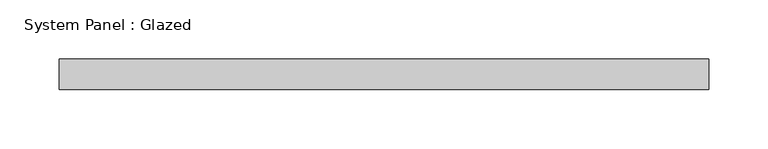
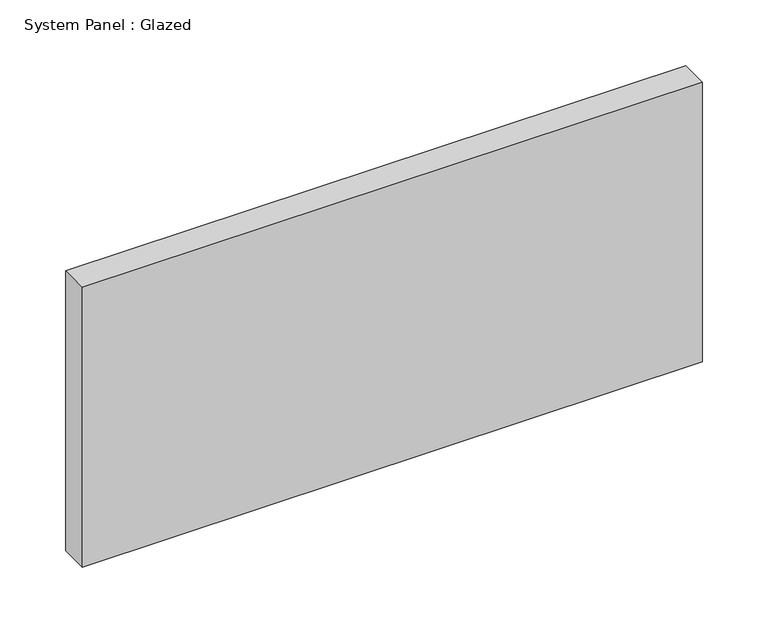
"""IFC4 building model written with IfcOpenShell, lengths in millimetres: plate geometry, System Panel : Glazed."""

from ifc_helpers import new_model, si_unit, origin, origin_with_axes, place, context, project, spatial, polyline, outline, extrude, source, transform, mapped, element, save


def system_panel_glazed_6ade1748(model_context):
    return source(origin(), model_context, "Body", "SweptSolid", [
        extrude(outline(polyline([(273.05, 19.05), (-273.05, 19.05), (-273.05, 44.45), (273.05, 44.45), (273.05, 19.05)])), origin_with_axes(), (0.0, 0.0, 1.0), 260.35),
    ])


if __name__ == "__main__":
    model = new_model("IFC4")
    model_context = context("Model", 3, world=origin())
    ifc_project = project(units=[si_unit("LENGTHUNIT", "METRE", prefix="MILLI")], contexts=[model_context])
    site = spatial("IfcSite", under=ifc_project)
    building = spatial("IfcBuilding", under=site)
    placement = place(None, origin())
    system_panel_glazed_shape = system_panel_glazed_6ade1748(model_context)
    element("IfcPlate", 1, ObjectType="System Panel : Glazed", at=placement, inside=building, context=model_context, shape_type="MappedRepresentation", body=[
        mapped(system_panel_glazed_shape, transform((0.0, 0.0, 0.0), x_axis=(1.0, 0.0, 0.0), y_axis=(0.0, 1.0, 0.0), z_axis=(0.0, 0.0, 1.0))),
    ])
    save(model, "model.ifc")

# Revit data of these elements
# Type "System Panel : Glazed"
#   Construction Type Id = "GSP4R"
#   Analytic Construction = "1/8 in Pilkington single glazing"
#   Visual Light Transmittance = 0.9
#   Solar Heat Gain Coefficient = 0.86
#   Heat Transfer Coefficient (U) = 1.18115 BTU/(h·ft²·°F)
#   Define Thermal Properties by = 1
# Element 1 (IfcPlate, "System Panel : Glazed")
#   Materials on its faces: "Glass"
# Materials
#   "Glass": class "Glass", colour RGB 0 128 192, transparency 0.75, Description = "Soda Lime Glass", Cost = 0
